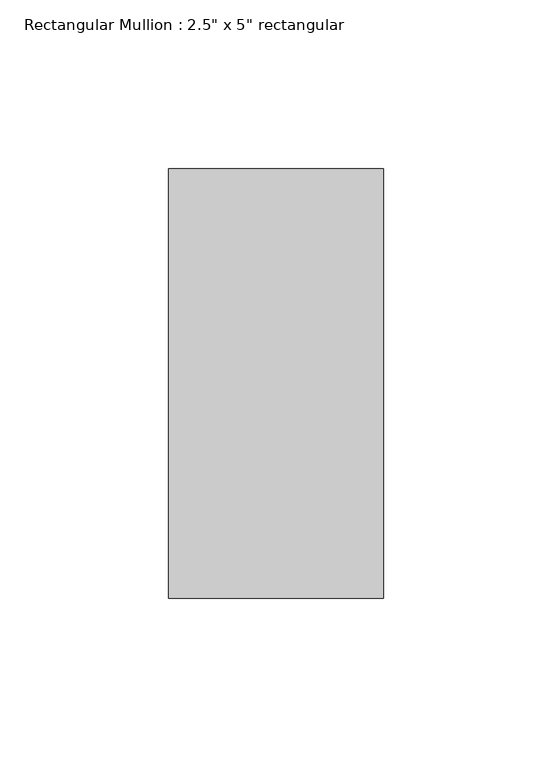
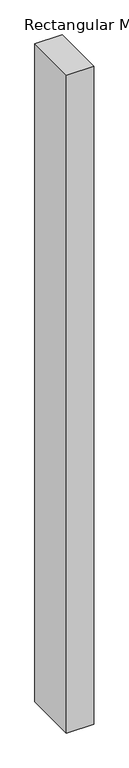
"""IFC4 building model written with IfcOpenShell, lengths in millimetres: member geometry."""

from ifc_helpers import new_model, si_unit, frame, origin, place, context, project, spatial, polyline, outline, extrude, source, transform, mapped, element, save


def member_40397874(model_context):
    return source(origin(), model_context, "Body", "SweptSolid", [
        extrude(outline(polyline([(0.0, 63.5), (0.0, -63.5), (-63.5, -63.5), (-63.5, 63.5), (0.0, 63.5)])), frame((0.0, 0.0, -1617.4100631), z_axis=(0.0, 0.0, 1.0), x_axis=(1.0, 0.0, 0.0)), (0.0, 0.0, 1.0), 1617.4100631),
    ])


if __name__ == "__main__":
    model = new_model("IFC4")
    model_context = context("Model", 3, world=origin())
    ifc_project = project(units=[si_unit("LENGTHUNIT", "METRE", prefix="MILLI")], contexts=[model_context])
    site = spatial("IfcSite", under=ifc_project)
    building = spatial("IfcBuilding", under=site)
    placement = place(None, origin())
    member_shape = member_40397874(model_context)
    element("IfcMember", 1, ObjectType="Rectangular Mullion : 2.5\" x 5\" rectangular", at=placement, inside=building, context=model_context, shape_type="MappedRepresentation", body=[
        mapped(member_shape, transform((0.0, 0.0, 0.0), x_axis=(1.0, 0.0, 0.0), y_axis=(0.0, 1.0, 0.0), z_axis=(0.0, 0.0, 1.0))),
    ])
    save(model, "model.ifc")

# Revit data of these elements
# Type "Rectangular Mullion : 2.5\" x 5\" rectangular"
#   built-in parameter 1007304 = 0.416667 (stored number, unit not read)
#   built-in parameter 1007301 = 0.104167 (stored number, unit not read)
#   built-in parameter 1007300 = 0.104167 (stored number, unit not read)
# Element 1 (IfcMember, "Rectangular Mullion : 2.5\" x 5\" rectangular")
#   Materials on its faces: "Aluminum"
# Materials
#   "Aluminum": class "Metal", colour RGB 247 247 247, transparency 0, Description = "Aluminum 6061", Cost = 0
